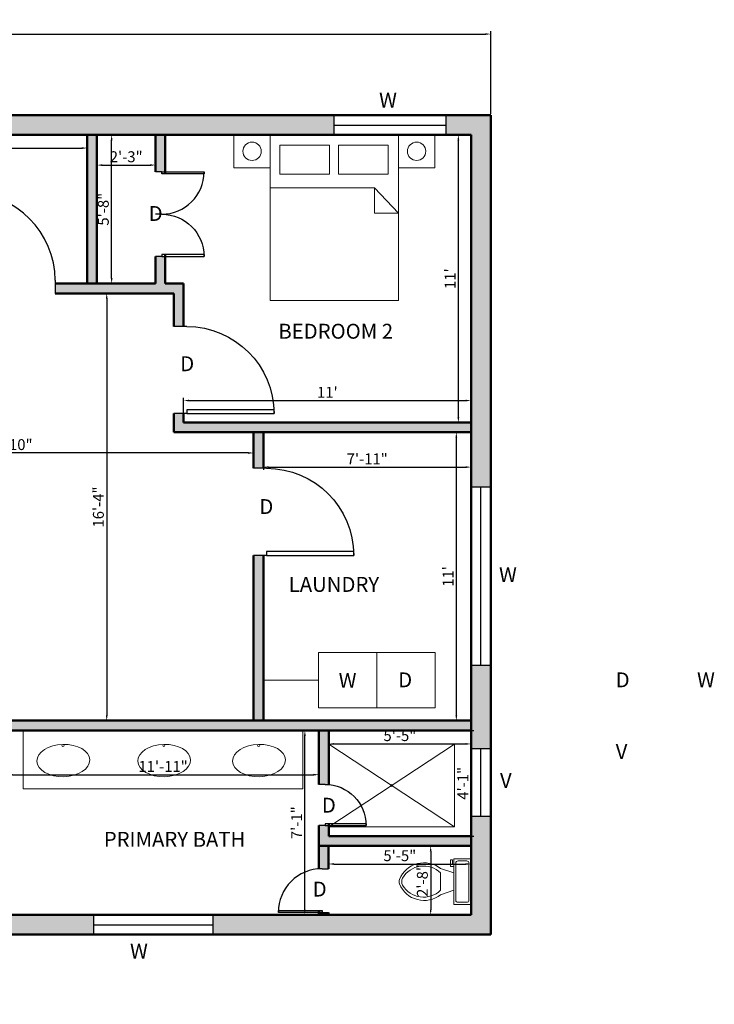
# Model space of a CAD drawing. Units: inches. Extents: x 1838 to 3464, y 573 to 2547.
# Tile 5 of 6: x 3055 to 3374, y 1336 to 1788. Entities that reach past the tile are written whole.
import ezdxf

# ---------------------------------------------------------------- set-up
doc = ezdxf.new("R2010")
doc.units = ezdxf.units.IN
for name, color, linetype, lineweight in [('A-ANNO-DIMS', 2, 'Continuous', 18), ('A-ANNO-TEXT', 7, 'Continuous', 18), ('A-AREA-IDEN', 3, 'Continuous', 18), ('A-DOOR', 4, 'Continuous', 25), ('A-EQPM', 9, 'Continuous', 18), ('A-FLOR-FIXT', 9, 'Continuous', 18), ('A-FURN', 8, 'Continuous', 18), ('A-GLAZ', 3, 'Continuous', 25), ('A-WALL', 1, 'Continuous', 50), ('A-WALL-PATT', 8, 'Continuous', 13)]:
    doc.layers.add(name, color=color, linetype=linetype, lineweight=lineweight)
doc.styles.get("Standard").update_dxf_attribs({"font": 'arial.ttf'})
doc.dimstyles.new('ISO-25', dxfattribs={"dimtxt": 5, "dimasz": 2.5, "dimexe": 1.25, "dimexo": 0.625, "dimtad": 1, "dimdec": 0, "dimlunit": 4, "dimtxsty": 'Standard', "dimcen": 2.5, "dimadec": 0, "dimazin": 0, "dimtfac": 1, "dimtdec": 0, "dimtmove": 0, "dimatfit": 3, "dimfxl": 1, "dimarcsym": 0})

# ---------------------------------------------------------------- blocks, each defined once
blk = doc.blocks.new('*U2')
for p, q in [((0, 0), (0, -6)), ((40, 0), (40, -6))]:
    blk.add_line(p, q)
blk.add_lwpolyline([(0, 0), (0, 40), (1.75, 40), (1.75, 0)], close=True)
blk.add_arc((0, 0), 40, 0, 90)
blk = doc.blocks.new('*U4')
for p, q in [((9.5, -6), (9.5, -2)), ((-10, -8.5), (-8, -8.5)), ((-10, -9.5), (-10, -8.5)), ((-8, -8.5), (-8, -8)), ((-7, -8), (-7, -9.5)), ((-4, -8), (-6, -14)), ((4, -8), (6, -14)), ((-7, -9.5), (-10, -9.5)), ((4, -14), (-4, -14))]:
    blk.add_line(p, q)
blk.add_lwpolyline([(10.5, -8), (10.5, 0), (-10.5, 0), (-10.5, -8)], close=True)
for points in [[(-9.5, -2), (-9.5, -6)], [(8.5, -1), (-8.5, -1)], [(-8.5, -7), (8.5, -7)]]:
    blk.add_lwpolyline(points)
for centre, radius, start, end in [((-8.62, -1.88), 0.884, 81.8699, 188.1301), ((8.62, -1.88), 0.884, 351.8699, 98.1301), ((-8.62, -6.12), 0.884, 171.8699, 278.1301), ((8.62, -6.12), 0.884, 261.8699, 8.1301), ((3.52, -21.58), 12.17, 141.4691, 247.9714), ((4.2, -21.82), 11.33, 136.3677, 238.9468), ((-3.52, -21.58), 12.17, 292.0284, 38.5307), ((-4.2, -21.82), 11.33, 301.053, 43.6321), ((0, -27.88), 4, 245.7318, 294.2682), ((0, -29), 4, 254.8605, 285.1395)]:
    blk.add_arc(centre, radius, start, end)
blk = doc.blocks.new('*D24')
at = {"layer": 'A-ANNO-DIMS', "color": 0, "lineweight": -2, "transparency": 16777216}
for p, q in [((2937.02, 1734.46), (2937.02, 1727.78)), ((3086.23, 1734.46), (3086.23, 1727.78)), ((2939.52, 1729.03), (3083.73, 1729.03))]:
    blk.add_line(p, q, dxfattribs=at)
at = {"layer": 'A-ANNO-DIMS', "color": 0, "lineweight": 100, "transparency": 16777216}
for points in [[(2939.52, 1729.44), (2939.52, 1728.61), (2937.02, 1729.03)], [(3083.73, 1729.44), (3083.73, 1728.61), (3086.23, 1729.03)]]:
    blk.add_solid(points, dxfattribs=at)
at = {"layer": 'Defpoints', "color": 0, "lineweight": 100, "transparency": 16777216}
for p in [(2937.02, 1735.09), (3086.23, 1735.09), (3086.23, 1729.03)]:
    blk.add_point(p, dxfattribs=at)
at = {"layer": 'A-ANNO-DIMS', "color": 0, "transparency": 16777216, "insert": (3011.63, 1732.2), "char_height": 5, "attachment_point": 5}
blk.add_mtext('12\'-5"', dxfattribs=at)
blk = doc.blocks.new('*D26')
at = {"layer": 'A-ANNO-DIMS', "color": 0, "lineweight": -2, "transparency": 16777216}
for p, q in [((3090.73, 1734.46), (3090.73, 1719.96)), ((3117.57, 1734.46), (3117.57, 1719.96)), ((3093.23, 1721.21), (3115.07, 1721.21))]:
    blk.add_line(p, q, dxfattribs=at)
at = {"layer": 'A-ANNO-DIMS', "color": 0, "lineweight": 100, "transparency": 16777216}
for points in [[(3093.23, 1721.63), (3093.23, 1720.79), (3090.73, 1721.21)], [(3115.07, 1721.63), (3115.07, 1720.79), (3117.57, 1721.21)]]:
    blk.add_solid(points, dxfattribs=at)
at = {"layer": 'Defpoints', "color": 0, "lineweight": 100, "transparency": 16777216}
for p in [(3090.73, 1735.09), (3117.57, 1735.09), (3117.57, 1721.21)]:
    blk.add_point(p, dxfattribs=at)
at = {"layer": 'A-ANNO-DIMS', "color": 0, "transparency": 16777216, "insert": (3104.15, 1724.39), "char_height": 5, "attachment_point": 5}
blk.add_mtext('2\'-3"', dxfattribs=at)
blk = doc.blocks.new('*D27')
at = {"layer": 'A-ANNO-DIMS', "color": 0, "lineweight": -2, "transparency": 16777216}
for p, q in [((3130.52, 1603.71), (3130.52, 1614.41)), ((3133.02, 1613.16), (3260.02, 1613.16)), ((3262.52, 1603.71), (3262.52, 1614.41))]:
    blk.add_line(p, q, dxfattribs=at)
at = {"layer": 'A-ANNO-DIMS', "color": 0, "lineweight": 100, "transparency": 16777216}
for points in [[(3133.02, 1613.57), (3133.02, 1612.74), (3130.52, 1613.16)], [(3260.02, 1613.57), (3260.02, 1612.74), (3262.52, 1613.16)]]:
    blk.add_solid(points, dxfattribs=at)
at = {"layer": 'Defpoints', "color": 0, "lineweight": 100, "transparency": 16777216}
for p in [(3262.52, 1613.16), (3130.52, 1603.09), (3262.52, 1603.09)]:
    blk.add_point(p, dxfattribs=at)
at = {"layer": 'A-ANNO-DIMS', "color": 0, "transparency": 16777216, "insert": (3196.52, 1616.29), "char_height": 5, "attachment_point": 5}
blk.add_mtext("11'", dxfattribs=at)
blk = doc.blocks.new('*D28')
at = {"layer": 'A-ANNO-DIMS', "color": 0, "lineweight": -2, "transparency": 16777216}
for p, q in [((3261.9, 1735.09), (3255.42, 1735.09)), ((3256.67, 1605.59), (3256.67, 1732.59)), ((3261.9, 1603.09), (3255.42, 1603.09))]:
    blk.add_line(p, q, dxfattribs=at)
at = {"layer": 'A-ANNO-DIMS', "color": 0, "lineweight": 100, "transparency": 16777216}
for points in [[(3256.25, 1732.59), (3257.09, 1732.59), (3256.67, 1735.09)], [(3256.25, 1605.59), (3257.09, 1605.59), (3256.67, 1603.09)]]:
    blk.add_solid(points, dxfattribs=at)
at = {"layer": 'Defpoints', "color": 0, "lineweight": 100, "transparency": 16777216}
for p in [(3256.67, 1735.09), (3262.52, 1735.09), (3262.52, 1603.09)]:
    blk.add_point(p, dxfattribs=at)
at = {"layer": 'A-ANNO-DIMS', "color": 0, "transparency": 16777216, "insert": (3253.53, 1669.09), "char_height": 5, "attachment_point": 5, "rotation": 90}
blk.add_mtext("11'", dxfattribs=at)
blk = doc.blocks.new('*D29')
at = {"layer": 'A-ANNO-DIMS', "color": 0, "lineweight": -2, "transparency": 16777216}
for p, q in [((3091.36, 1735.09), (3098.71, 1735.09)), ((3097.46, 1669.34), (3097.46, 1732.59)), ((3091.36, 1666.84), (3098.71, 1666.84))]:
    blk.add_line(p, q, dxfattribs=at)
at = {"layer": 'A-ANNO-DIMS', "color": 0, "lineweight": 100, "transparency": 16777216}
for points in [[(3097.05, 1732.59), (3097.88, 1732.59), (3097.46, 1735.09)], [(3097.05, 1669.34), (3097.88, 1669.34), (3097.46, 1666.84)]]:
    blk.add_solid(points, dxfattribs=at)
at = {"layer": 'Defpoints', "color": 0, "lineweight": 100, "transparency": 16777216}
for p in [(3090.73, 1735.09), (3097.46, 1735.09), (3090.73, 1666.84)]:
    blk.add_point(p, dxfattribs=at)
at = {"layer": 'A-ANNO-DIMS', "color": 0, "transparency": 16777216, "insert": (3094.28, 1700.96), "char_height": 5, "attachment_point": 5, "rotation": 90}
blk.add_mtext('5\'-8"', dxfattribs=at)
blk = doc.blocks.new('*D30')
at = {"layer": 'A-ANNO-DIMS', "color": 0, "lineweight": -2, "transparency": 16777216}
for p, q in [((3167.14, 1597.96), (3167.14, 1581.36)), ((3262.52, 1597.96), (3262.52, 1581.36)), ((3169.64, 1582.61), (3260.02, 1582.61))]:
    blk.add_line(p, q, dxfattribs=at)
at = {"layer": 'A-ANNO-DIMS', "color": 0, "lineweight": 100, "transparency": 16777216}
for points in [[(3169.64, 1583.03), (3169.64, 1582.19), (3167.14, 1582.61)], [(3260.02, 1583.03), (3260.02, 1582.19), (3262.52, 1582.61)]]:
    blk.add_solid(points, dxfattribs=at)
at = {"layer": 'Defpoints', "color": 0, "lineweight": 100, "transparency": 16777216}
for p in [(3167.14, 1598.59), (3262.52, 1598.59), (3262.52, 1582.61)]:
    blk.add_point(p, dxfattribs=at)
at = {"layer": 'A-ANNO-DIMS', "color": 0, "transparency": 16777216, "insert": (3214.83, 1585.74), "char_height": 5, "attachment_point": 5}
blk.add_mtext('7\'-11"', dxfattribs=at)
blk = doc.blocks.new('*D31')
at = {"layer": 'A-ANNO-DIMS', "color": 0, "lineweight": -2, "transparency": 16777216}
for p, q in [((3261.9, 1598.59), (3254.49, 1598.59)), ((3255.74, 1596.09), (3255.74, 1468.77)), ((3261.9, 1466.27), (3254.49, 1466.27))]:
    blk.add_line(p, q, dxfattribs=at)
at = {"layer": 'A-ANNO-DIMS', "color": 0, "lineweight": 100, "transparency": 16777216}
for points in [[(3255.33, 1596.09), (3256.16, 1596.09), (3255.74, 1598.59)], [(3255.33, 1468.77), (3256.16, 1468.77), (3255.74, 1466.27)]]:
    blk.add_solid(points, dxfattribs=at)
at = {"layer": 'Defpoints', "color": 0, "lineweight": 100, "transparency": 16777216}
for p in [(3262.52, 1598.59), (3255.74, 1466.27), (3262.52, 1466.27)]:
    blk.add_point(p, dxfattribs=at)
at = {"layer": 'A-ANNO-DIMS', "color": 0, "transparency": 16777216, "insert": (3252.61, 1532.43), "char_height": 5, "attachment_point": 5, "rotation": 90}
blk.add_mtext("11'", dxfattribs=at)
blk = doc.blocks.new('*D32')
at = {"layer": 'A-ANNO-DIMS', "color": 0, "lineweight": -2, "transparency": 16777216}
for p, q in [((3261.9, 1408.74), (3242.71, 1408.74)), ((3243.96, 1406.24), (3243.96, 1379.59)), ((3261.9, 1377.09), (3242.71, 1377.09))]:
    blk.add_line(p, q, dxfattribs=at)
at = {"layer": 'A-ANNO-DIMS', "color": 0, "lineweight": 100, "transparency": 16777216}
for points in [[(3243.55, 1406.24), (3244.38, 1406.24), (3243.96, 1408.74)], [(3243.55, 1379.59), (3244.38, 1379.59), (3243.96, 1377.09)]]:
    blk.add_solid(points, dxfattribs=at)
at = {"layer": 'Defpoints', "color": 0, "lineweight": 100, "transparency": 16777216}
for p in [(3262.52, 1408.74), (3243.96, 1377.09), (3262.52, 1377.09)]:
    blk.add_point(p, dxfattribs=at)
at = {"layer": 'A-ANNO-DIMS', "color": 0, "transparency": 16777216, "insert": (3240.78, 1392.91), "char_height": 5, "attachment_point": 5, "rotation": 90}
blk.add_mtext('2\'-8"', dxfattribs=at)
blk = doc.blocks.new('*D33')
at = {"layer": 'A-ANNO-DIMS', "color": 0, "lineweight": -2, "transparency": 16777216}
for p, q in [((3197.06, 1408.11), (3197.06, 1399.22)), ((3262.52, 1408.11), (3262.52, 1399.22)), ((3199.56, 1400.47), (3260.02, 1400.47))]:
    blk.add_line(p, q, dxfattribs=at)
at = {"layer": 'A-ANNO-DIMS', "color": 0, "lineweight": 100, "transparency": 16777216}
for points in [[(3199.56, 1400.89), (3199.56, 1400.06), (3197.06, 1400.47)], [(3260.02, 1400.89), (3260.02, 1400.06), (3262.52, 1400.47)]]:
    blk.add_solid(points, dxfattribs=at)
at = {"layer": 'Defpoints', "color": 0, "lineweight": 100, "transparency": 16777216}
for p in [(3197.06, 1408.74), (3262.52, 1408.74), (3262.52, 1400.47)]:
    blk.add_point(p, dxfattribs=at)
at = {"layer": 'A-ANNO-DIMS', "color": 0, "transparency": 16777216, "insert": (3229.79, 1403.64), "char_height": 5, "attachment_point": 5}
blk.add_mtext('5\'-5"', dxfattribs=at)
blk = doc.blocks.new('*D34')
at = {"layer": 'A-ANNO-DIMS', "color": 0, "lineweight": -2, "transparency": 16777216}
for p, q in [((3263.15, 1461.77), (3263.77, 1461.77)), ((3262.52, 1415.74), (3262.52, 1459.27)), ((3263.15, 1413.24), (3263.77, 1413.24))]:
    blk.add_line(p, q, dxfattribs=at)
at = {"layer": 'A-ANNO-DIMS', "color": 0, "lineweight": 100, "transparency": 16777216}
for points in [[(3262.11, 1459.27), (3262.94, 1459.27), (3262.52, 1461.77)], [(3262.11, 1415.74), (3262.94, 1415.74), (3262.52, 1413.24)]]:
    blk.add_solid(points, dxfattribs=at)
at = {"layer": 'Defpoints', "color": 0, "lineweight": 100, "transparency": 16777216}
for p in [(3262.52, 1461.77), (3262.52, 1461.77), (3262.52, 1413.24)]:
    blk.add_point(p, dxfattribs=at)
at = {"layer": 'A-ANNO-DIMS', "color": 0, "transparency": 16777216, "insert": (3259.39, 1437.5), "char_height": 5, "attachment_point": 5, "rotation": 90}
blk.add_mtext('4\'-1"', dxfattribs=at)
blk = doc.blocks.new('*D35')
at = {"layer": 'A-ANNO-DIMS', "color": 0, "lineweight": -2, "transparency": 16777216}
for p, q in [((3197.12, 1461.14), (3197.12, 1454.32)), ((3262.52, 1461.14), (3262.52, 1454.32)), ((3199.62, 1455.57), (3260.02, 1455.57))]:
    blk.add_line(p, q, dxfattribs=at)
at = {"layer": 'A-ANNO-DIMS', "color": 0, "lineweight": 100, "transparency": 16777216}
for points in [[(3199.62, 1455.99), (3199.62, 1455.16), (3197.12, 1455.57)], [(3260.02, 1455.99), (3260.02, 1455.16), (3262.52, 1455.57)]]:
    blk.add_solid(points, dxfattribs=at)
at = {"layer": 'Defpoints', "color": 0, "lineweight": 100, "transparency": 16777216}
for p in [(3197.12, 1461.77), (3262.52, 1461.77), (3262.52, 1455.57)]:
    blk.add_point(p, dxfattribs=at)
at = {"layer": 'A-ANNO-DIMS', "color": 0, "transparency": 16777216, "insert": (3229.82, 1458.74), "char_height": 5, "attachment_point": 5}
blk.add_mtext('5\'-5"', dxfattribs=at)
blk = doc.blocks.new('*D36')
at = {"layer": 'A-ANNO-DIMS', "color": 0, "lineweight": -2, "transparency": 16777216}
for p, q in [((3049.57, 1461.14), (3049.57, 1440.21)), ((3192.62, 1461.14), (3192.62, 1440.21)), ((3052.07, 1441.46), (3190.12, 1441.46))]:
    blk.add_line(p, q, dxfattribs=at)
at = {"layer": 'A-ANNO-DIMS', "color": 0, "lineweight": 100, "transparency": 16777216}
for points in [[(3052.07, 1441.87), (3052.07, 1441.04), (3049.57, 1441.46)], [(3190.12, 1441.87), (3190.12, 1441.04), (3192.62, 1441.46)]]:
    blk.add_solid(points, dxfattribs=at)
at = {"layer": 'Defpoints', "color": 0, "lineweight": 100, "transparency": 16777216}
for p in [(3049.57, 1461.77), (3192.62, 1461.77), (3192.62, 1441.46)]:
    blk.add_point(p, dxfattribs=at)
at = {"layer": 'A-ANNO-DIMS', "color": 0, "transparency": 16777216, "insert": (3121.09, 1444.59), "char_height": 5, "attachment_point": 5}
blk.add_mtext('11\'-11"', dxfattribs=at)
blk = doc.blocks.new('*D37')
at = {"layer": 'A-ANNO-DIMS', "color": 0, "lineweight": -2, "transparency": 16777216}
for p, q in [((3191.99, 1461.77), (3184.93, 1461.77)), ((3186.18, 1379.59), (3186.18, 1459.27)), ((3191.99, 1377.09), (3184.93, 1377.09))]:
    blk.add_line(p, q, dxfattribs=at)
at = {"layer": 'A-ANNO-DIMS', "color": 0, "lineweight": 100, "transparency": 16777216}
for points in [[(3185.77, 1459.27), (3186.6, 1459.27), (3186.18, 1461.77)], [(3185.77, 1379.59), (3186.6, 1379.59), (3186.18, 1377.09)]]:
    blk.add_solid(points, dxfattribs=at)
at = {"layer": 'Defpoints', "color": 0, "lineweight": 100, "transparency": 16777216}
for p in [(3186.18, 1461.77), (3192.62, 1461.77), (3192.62, 1377.09)]:
    blk.add_point(p, dxfattribs=at)
at = {"layer": 'A-ANNO-DIMS', "color": 0, "transparency": 16777216, "insert": (3183.05, 1419.43), "char_height": 5, "attachment_point": 5, "rotation": 90}
blk.add_mtext('7\'-1"', dxfattribs=at)
blk = doc.blocks.new('*D50')
at = {"layer": 'A-ANNO-DIMS', "color": 0, "lineweight": -2, "transparency": 16777216}
for p, q in [((2937.02, 1597.96), (2937.02, 1587.86)), ((3162.64, 1597.96), (3162.64, 1587.86)), ((3160.14, 1589.11), (2939.52, 1589.11))]:
    blk.add_line(p, q, dxfattribs=at)
at = {"layer": 'A-ANNO-DIMS', "color": 0, "lineweight": 100, "transparency": 16777216}
for points in [[(2939.52, 1589.52), (2939.52, 1588.69), (2937.02, 1589.11)], [(3160.14, 1589.52), (3160.14, 1588.69), (3162.64, 1589.11)]]:
    blk.add_solid(points, dxfattribs=at)
at = {"layer": 'Defpoints', "color": 0, "lineweight": 100, "transparency": 16777216}
for p in [(2937.02, 1598.59), (3162.64, 1598.59), (2937.02, 1589.11)]:
    blk.add_point(p, dxfattribs=at)
at = {"layer": 'A-ANNO-DIMS', "color": 0, "transparency": 16777216, "insert": (3049.83, 1592.29), "char_height": 5, "attachment_point": 5}
blk.add_mtext('18\'-10"', dxfattribs=at)
blk = doc.blocks.new('*D51')
at = {"layer": 'A-ANNO-DIMS', "color": 0, "lineweight": -2, "transparency": 16777216}
for p, q in [((3125.4, 1662.34), (3093.94, 1662.34)), ((3095.19, 1659.84), (3095.19, 1468.77)), ((3125.4, 1466.27), (3093.94, 1466.27))]:
    blk.add_line(p, q, dxfattribs=at)
at = {"layer": 'A-ANNO-DIMS', "color": 0, "lineweight": 100, "transparency": 16777216}
for points in [[(3094.77, 1659.84), (3095.61, 1659.84), (3095.19, 1662.34)], [(3094.77, 1468.77), (3095.61, 1468.77), (3095.19, 1466.27)]]:
    blk.add_solid(points, dxfattribs=at)
at = {"layer": 'Defpoints', "color": 0, "lineweight": 100, "transparency": 16777216}
for p in [(3126.02, 1662.34), (3095.19, 1466.27), (3126.02, 1466.27)]:
    blk.add_point(p, dxfattribs=at)
at = {"layer": 'A-ANNO-DIMS', "color": 0, "transparency": 16777216, "insert": (3092.01, 1564.3), "char_height": 5, "attachment_point": 5, "rotation": 90}
blk.add_mtext('16\'-4"', dxfattribs=at)
blk = doc.blocks.new('*D65')
at = {"layer": 'A-ANNO-DIMS', "color": 0, "lineweight": -2, "transparency": 16777216}
for p, q in [((2791.52, 1744.71), (2791.52, 1782.6)), ((2794.02, 1781.35), (3269.02, 1781.35)), ((3271.52, 1744.71), (3271.52, 1782.6))]:
    blk.add_line(p, q, dxfattribs=at)
at = {"layer": 'A-ANNO-DIMS', "color": 0, "lineweight": 100, "transparency": 16777216}
for points in [[(2794.02, 1781.77), (2794.02, 1780.94), (2791.52, 1781.35)], [(3269.02, 1781.77), (3269.02, 1780.94), (3271.52, 1781.35)]]:
    blk.add_solid(points, dxfattribs=at)
at = {"layer": 'Defpoints', "color": 0, "lineweight": 100, "transparency": 16777216}
for p in [(3271.52, 1781.35), (2791.52, 1744.09), (3271.52, 1744.09)]:
    blk.add_point(p, dxfattribs=at)
at = {"layer": 'A-ANNO-DIMS', "color": 0, "transparency": 16777216, "insert": (3031.52, 1784.53), "char_height": 5, "attachment_point": 5}
blk.add_mtext("40'", dxfattribs=at)
blk = doc.blocks.new('BED-QUEEN')
for p, q in [((2829.57, 1710.8), (2877.39, 1710.8)), ((2877.39, 1710.8), (2877.39, 1699.19)), ((2888.43, 1699.19), (2877.39, 1710.8)), ((2877.39, 1699.19), (2888.43, 1699.19))]:
    blk.add_line(p, q)
for points in [[(2829.57, 1735.09), (2812.9, 1735.09), (2812.9, 1719.98), (2829.57, 1719.98)], [(2829.57, 1735.09), (2888.43, 1735.09), (2888.43, 1659.13), (2829.57, 1659.13)], [(2905.11, 1735.09), (2888.43, 1735.09), (2888.43, 1719.98), (2905.11, 1719.98)]]:
    blk.add_lwpolyline(points, close=True)
for centre in [(2821.24, 1727.53), (2896.77, 1727.53)]:
    blk.add_circle(centre, 4.22)

msp = doc.modelspace()

# ---------------------------------------------------------------- hatches: boundary and pattern name
at = {"layer": 'A-WALL-PATT'}
h = msp.add_hatch(color=256, dxfattribs=at)
h.dxf.hatch_style = 1
h.paths.add_polyline_path([(2800.52, 1735.09), (2834.76, 1735.09), (2834.76, 1744.09), (2791.52, 1744.09), (2791.52, 1591.27), (2800.52, 1591.27)])
h.paths.add_polyline_path([(2982.96, 1744.09), (2885.93, 1744.09), (2885.93, 1735.09), (2888.43, 1735.09), (2932.52, 1735.09), (2982.96, 1735.09)])
h.paths.add_polyline_path([(3199.72, 1744.09), (3031.52, 1744.09), (3031.52, 1735.09), (3199.72, 1735.09)])
h.paths.add_polyline_path([(3271.52, 1744.09), (3250.89, 1744.09), (3250.89, 1735.09), (3262.52, 1735.09), (3262.52, 1573.47), (3271.52, 1573.47)])
h.paths.add_polyline_path([(3262.52, 1603.09), (3130.52, 1603.09), (3130.52, 1607.14), (3126.02, 1607.14), (3126.02, 1598.59), (3262.52, 1598.59)])
h.paths.add_polyline_path([(3130.52, 1666.84), (3122.07, 1666.84), (3122.07, 1679.27), (3120.48, 1679.27), (3117.57, 1679.27), (3117.57, 1666.84), (3071.52, 1666.84), (3071.52, 1662.34), (3126.02, 1662.34), (3126.02, 1647.14), (3130.52, 1647.14)])
h.paths.add_polyline_path([(3122.07, 1735.09), (3117.57, 1735.09), (3117.57, 1718.07), (3120.48, 1718.07), (3122.07, 1718.07)])
h.paths.add_polyline_path([(3090.73, 1735.09), (3086.23, 1735.09), (3086.23, 1666.84), (3090.73, 1666.84)])
h.paths.add_polyline_path([(3031.52, 1666.84), (2937.02, 1666.84), (2937.02, 1662.34), (3031.52, 1662.34)])
h.paths.add_polyline_path([(2937.02, 1735.09), (2932.52, 1735.09), (2932.52, 1646.12), (2937.02, 1646.12)])
h.paths.add_polyline_path([(2937.02, 1606.12), (2932.52, 1606.12), (2932.52, 1603.09), (2852.18, 1603.09), (2852.18, 1598.59), (2937.02, 1598.59)])
h.paths.add_polyline_path([(2852.18, 1603.09), (2845.88, 1603.09), (2845.88, 1601.49), (2845.88, 1598.59), (2852.18, 1598.59)])
h.paths.add_polyline_path([(2807.08, 1601.49), (2807.08, 1603.09), (2800.52, 1603.09), (2800.52, 1598.59), (2807.08, 1598.59)], flags=17)
h.paths.add_polyline_path([(2937.02, 1598.59), (2932.24, 1598.59), (2932.24, 1570.68), (2937.02, 1570.68)])
h.paths.add_polyline_path([(2800.52, 1513.09), (2800.52, 1533.8), (2791.52, 1533.8), (2791.52, 1336.09), (2852.63, 1336.09), (2852.63, 1345.09), (2840.19, 1345.09), (2823.52, 1345.09), (2800.52, 1345.09)])
h.paths.add_polyline_path([(2807.08, 1472.56), (2807.08, 1475.47), (2800.52, 1475.47), (2800.52, 1470.97), (2807.08, 1470.97)], flags=17)
h.paths.add_polyline_path([(2892.01, 1513.09), (2887.51, 1513.09), (2887.51, 1475.47), (2845.88, 1475.47), (2845.88, 1472.56), (2845.88, 1470.97), (2892.01, 1470.97)])
h.paths.add_polyline_path([(2973.02, 1517.59), (2800.52, 1517.59), (2800.52, 1513.09), (2968.52, 1513.09), (2968.52, 1510.98), (2973.02, 1510.98)])
h.paths.add_polyline_path([(2856.68, 1598.59), (2852.18, 1598.59), (2852.18, 1517.59), (2856.68, 1517.59)])
h.paths.add_polyline_path([(2973.02, 1376.09), (2973.02, 1377.09), (2968.52, 1377.09), (2968.52, 1345.09), (2903.8, 1345.09), (2903.8, 1336.09), (2973.02, 1336.09)])
h.paths.add_polyline_path([(3089.35, 1377.09), (2973.02, 1377.09), (2973.02, 1368.09), (3089.35, 1368.09)])
h.paths.add_polyline_path([(2973.02, 1470.98), (2968.52, 1470.98), (2968.52, 1398.48), (2973.02, 1398.48)])
h.paths.add_polyline_path([(3262.52, 1466.27), (2973.02, 1466.27), (2973.02, 1461.77), (3262.52, 1461.77)])
h.paths.add_polyline_path([(3017.96, 1406), (3045.44, 1406), (3045.44, 1404.8), (3017.93, 1404.8), (3017.93, 1406), (3017.96, 1406, -0.397522), (3045.07, 1432.31), (3045.07, 1461.77), (3049.57, 1461.77), (3049.57, 1432.31), (3045.44, 1432.31, 0.401453)])
h.paths.add_polyline_path([(3049.57, 1404.8), (3045.07, 1404.8), (3045.07, 1402.98), (2973.02, 1402.98), (2973.02, 1398.48), (3049.57, 1398.48)])
h.paths.add_polyline_path([(3271.52, 1422.39), (3262.52, 1422.39), (3262.52, 1377.09), (3143.98, 1377.09), (3143.98, 1368.09), (3271.52, 1368.09)])
h.paths.add_polyline_path([(3271.52, 1491.77), (3262.52, 1491.77), (3262.52, 1453.4), (3271.52, 1453.4)])
h.paths.add_polyline_path([(3167.14, 1542.08), (3162.64, 1542.08), (3162.64, 1466.27), (3167.14, 1466.27)])
h.paths.add_polyline_path([(3167.14, 1598.59), (3162.64, 1598.59), (3162.64, 1582.08), (3167.14, 1582.08)])
h = msp.add_hatch(color=256, dxfattribs=at)
h.dxf.hatch_style = 1
h.paths.add_polyline_path([(3197.12, 1461.77), (3192.62, 1461.77), (3192.62, 1436.99), (3195.45, 1436.99, -0.022103), (3197.12, 1436.92)])
h.paths.add_polyline_path([(3262.52, 1413.24), (3197.12, 1413.24), (3197.12, 1418.11), (3195.45, 1418.11), (3192.62, 1418.11), (3192.62, 1408.74), (3262.52, 1408.74)])
h.paths.add_polyline_path([(3197.06, 1408.74), (3192.62, 1408.74), (3192.62, 1398.28, -0.017972), (3194.06, 1398.33), (3197.06, 1398.33)])
h = msp.add_hatch(color=256, dxfattribs=at)
h.dxf.hatch_style = 1
h.paths.add_polyline_path([(3197.06, 1378.28), (3194.06, 1378.28), (3192.62, 1378.28), (3192.62, 1377.09), (3197.06, 1377.09)])

# ---------------------------------------------------------------- linework, layer by layer
at = {"layer": 'A-EQPM'}
for p, q in [((3219.26, 1472.07), (3219.26, 1497.55)), ((3192.52, 1484.81), (3167.14, 1484.81))]:
    msp.add_line(p, q, dxfattribs=at)
msp.add_lwpolyline([(3192.52, 1472.07), (3246, 1472.07), (3246, 1497.55), (3192.52, 1497.55)], close=True, dxfattribs=at)
at = {"layer": 'A-FLOR-FIXT'}
for p, q in [((3197.12, 1455.49), (3254.92, 1455.49)), ((3197.12, 1417.56), (3254.92, 1455.49)), ((3254.92, 1417.56), (3197.12, 1455.49)), ((3254.92, 1455.49), (3254.92, 1417.56)), ((3254.92, 1417.56), (3197.12, 1417.56))]:
    msp.add_line(p, q, dxfattribs=at)
msp.add_lwpolyline([(3056.84, 1461.77), (3185.21, 1461.77), (3185.21, 1434.97), (3056.84, 1434.97)], close=True, dxfattribs=at)
for centre, radius in [((3075.11, 1454.9), 0.474), ((3121.42, 1454.9), 0.474), ((3164.96, 1454.9), 0.474), ((3226.02, 1436.52), 0.409)]:
    msp.add_circle(centre, radius, dxfattribs=at)
for centre in [(3075.27, 1447.95), (3121.58, 1447.95), (3165.13, 1447.95)]:
    msp.add_ellipse(centre, major_axis=(12.1, 0.29), ratio=0.613887, dxfattribs=at)
at = {"layer": 'A-FURN'}
for points in [[(3174.62, 1730.28), (3197.49, 1730.28), (3197.49, 1716.98), (3174.62, 1716.98)], [(3201.61, 1730.28), (3224.48, 1730.28), (3224.48, 1716.98), (3201.61, 1716.98)]]:
    msp.add_lwpolyline(points, close=True, dxfattribs=at)
at = {"layer": 'A-GLAZ'}
for p, q in [((3199.72, 1739.59), (3250.89, 1739.59)), ((3267.02, 1491.77), (3267.02, 1573.47)), ((3267.02, 1422.39), (3267.02, 1453.4)), ((3089.35, 1372.59), (3143.98, 1372.59))]:
    msp.add_line(p, q, dxfattribs=at)
for points in [[(3199.72, 1744.09), (3250.89, 1744.09), (3250.89, 1735.09), (3199.72, 1735.09)], [(3262.52, 1491.77), (3271.52, 1491.77), (3271.52, 1573.47), (3262.52, 1573.47)], [(3262.52, 1422.39), (3271.52, 1422.39), (3271.52, 1453.4), (3262.52, 1453.4)], [(3143.98, 1368.09), (3089.35, 1368.09), (3089.35, 1377.09), (3143.98, 1377.09)]]:
    msp.add_lwpolyline(points, close=True, dxfattribs=at)
at = {"layer": 'A-WALL'}
for p, q in [((2791.52, 1744.09), (3271.52, 1744.09)), ((3271.52, 1744.09), (3271.52, 1368.09)), ((2800.52, 1735.09), (3262.52, 1735.09)), ((3086.23, 1735.09), (3086.23, 1666.84)), ((3090.73, 1735.09), (3090.73, 1666.84)), ((3117.57, 1718.07), (3117.57, 1735.09)), ((3122.07, 1717.22), (3122.07, 1735.09)), ((3262.52, 1735.09), (3130.52, 1735.09)), ((3262.52, 1735.09), (3262.52, 1377.09)), ((3122.07, 1698.6), (3122.07, 1698.73)), ((3117.57, 1666.84), (3117.57, 1679.27)), ((3122.07, 1666.84), (3122.07, 1680.12)), ((3117.57, 1666.84), (3071.52, 1666.84)), ((3130.52, 1666.84), (3122.07, 1666.84)), ((3130.52, 1666.84), (3130.52, 1647.14)), ((3126.02, 1662.34), (3071.52, 1662.34)), ((3126.02, 1662.34), (3126.02, 1647.14)), ((3126.02, 1607.14), (3126.02, 1598.59)), ((3130.52, 1607.14), (3130.52, 1603.09)), ((3130.52, 1603.09), (3262.52, 1603.09)), ((3126.02, 1598.59), (3262.52, 1598.59)), ((3162.64, 1598.59), (3162.64, 1582.08)), ((3167.14, 1598.59), (3167.14, 1582.08)), ((3162.64, 1542.08), (3162.64, 1466.27)), ((3167.14, 1542.08), (3167.14, 1466.27)), ((2973.02, 1466.27), (3262.52, 1466.27)), ((2973.02, 1461.77), (3262.52, 1461.77)), ((3192.62, 1461.77), (3192.62, 1436.99)), ((3197.12, 1461.77), (3197.12, 1436.92)), ((3197.12, 1455.49), (3197.12, 1455.49)), ((3197.12, 1418.93), (3197.12, 1413.24)), ((3192.62, 1418.11), (3192.62, 1408.74)), ((3197.12, 1413.24), (3262.52, 1413.24)), ((3192.62, 1408.74), (3262.52, 1408.74)), ((3192.62, 1408.74), (3192.62, 1398.28)), ((3197.06, 1408.74), (3197.06, 1398.33)), ((3192.62, 1379.16), (3192.62, 1377.09)), ((3197.06, 1378.28), (3197.06, 1377.09)), ((2973.02, 1377.09), (3262.52, 1377.09)), ((2973.02, 1368.09), (3271.52, 1368.09))]:
    msp.add_line(p, q, dxfattribs=at)

# ---------------------------------------------------------------- block references
at = {"layer": 'A-DOOR'}
for p, xscale, yscale, zscale, rotation in [((3120.48, 1718.07), 0.4849649576214688, 0.4849649576214688, 0.4849649576214688, 270), ((3120.48, 1679.27), -0.4849649576214688, 0.4849649576214688, 0.4849649576214688, 270), ((3195.45, 1418.11), -0.4721246961780511, 0.4721246961780511, 0.4721246961780511, 270), ((3194.06, 1378.28), 0.5010716583969415, 0.5010716583969415, 0.5010716583969415, 90)]:
    msp.add_blockref('*U2', p, dxfattribs=dict(at, xscale=xscale, yscale=yscale, zscale=zscale, rotation=rotation))
msp.add_blockref('*U2', (3031.52, 1668.34), dxfattribs=at)
at = {"layer": 'A-DOOR', "xscale": -1, "rotation": 270}
for p in [(3132.02, 1607.14), (3168.64, 1542.08)]:
    msp.add_blockref('*U2', p, dxfattribs=at)
at = {"layer": 'A-FLOR-FIXT', "rotation": 270}
msp.add_blockref('*U4', (3262.52, 1392.39), dxfattribs=at)
at = {"layer": 'A-FURN'}
msp.add_blockref('BED-QUEEN', (340.72, 0), dxfattribs=at)

# ---------------------------------------------------------------- texts
at = {"layer": 'A-ANNO-TEXT', "char_height": 6.84, "attachment_point": 1}
for s, insert in [('W', (3220.27, 1754.47)), ('D', (3114.46, 1702.42)), ('D', (3128.96, 1633.47)), ('D', (3165.3, 1567.92)), ('W', (3275.34, 1536.67)), ('W', (3201.7, 1488.16)), ('D', (3229.06, 1488.39)), ('D', (3328.92, 1488.39)), ('W', (3366.27, 1488.39)), ('V', (3328.92, 1455.54)), ('V', (3275.79, 1442.26)), ('D', (3194, 1430.87)), ('D', (3189.79, 1392.37)), ('W', (3105.89, 1363.93))]:
    msp.add_mtext_dynamic_manual_height_columns(s, width=95.5762, gutter_width=34.2, heights=[0], dxfattribs=dict(at, insert=insert))
at = {"layer": 'A-AREA-IDEN', "attachment_point": 1}
for s, insert, char_height in [('BEDROOM 2', (3174.03, 1648.38), 6.841), ('LAUNDRY', (3178.78, 1532.2), 6.841), ('PRIMARY BATH', (3093.86, 1415.21), 6.8407)]:
    msp.add_mtext_dynamic_manual_height_columns(s, width=95.5762, gutter_width=34.2, heights=[0], dxfattribs=dict(at, insert=insert, char_height=char_height))

# ---------------------------------------------------------------- dimensions: what is measured, and where the dimension line sits
at = {"layer": 'A-ANNO-DIMS'}
for base, p1, p2, picture, middle in [((3271.52, 1781.35), (2791.52, 1744.09), (3271.52, 1744.09), '*D65', (3031.52, 1784.53)), ((3086.23, 1729.03), (2937.02, 1735.09), (3086.23, 1735.09), '*D24', (3011.63, 1732.2)), ((3117.57, 1721.21), (3090.73, 1735.09), (3117.57, 1735.09), '*D26', (3104.15, 1724.39)), ((3262.52, 1613.16), (3130.52, 1603.09), (3262.52, 1603.09), '*D27', (3196.52, 1616.29)), ((2937.02, 1589.11), (3162.64, 1598.59), (2937.02, 1598.59), '*D50', (3049.83, 1592.29)), ((3262.52, 1582.61), (3167.14, 1598.59), (3262.52, 1598.59), '*D30', (3214.83, 1585.74)), ((3192.62, 1441.46), (3049.57, 1461.77), (3192.62, 1461.77), '*D36', (3121.09, 1444.59)), ((3262.52, 1455.57), (3197.12, 1461.77), (3262.52, 1461.77), '*D35', (3229.82, 1458.74)), ((3262.52, 1400.47), (3197.06, 1408.74), (3262.52, 1408.74), '*D33', (3229.79, 1403.64))]:
    dim = msp.add_linear_dim(base=base, p1=p1, p2=p2, dimstyle='ISO-25', override={"dimclrd": 0, "dimclre": 0, "dimclrt": 0}, dxfattribs=at)
    dim.commit()
    dim.dimension.update_dxf_attribs({"geometry": picture, "text_midpoint": middle})
for base, p1, p2, picture, middle in [((3097.46, 1735.09), (3090.73, 1666.84), (3090.73, 1735.09), '*D29', (3094.28, 1700.96)), ((3256.67, 1735.09), (3262.52, 1603.09), (3262.52, 1735.09), '*D28', (3253.53, 1669.09)), ((3095.19, 1466.27), (3126.02, 1662.34), (3126.02, 1466.27), '*D51', (3092.01, 1564.3)), ((3255.74, 1466.27), (3262.52, 1598.59), (3262.52, 1466.27), '*D31', (3252.61, 1532.43)), ((3186.18, 1461.77), (3192.62, 1377.09), (3192.62, 1461.77), '*D37', (3183.05, 1419.43)), ((3262.52, 1461.77), (3262.52, 1413.24), (3262.52, 1461.77), '*D34', (3259.39, 1437.5)), ((3243.96, 1377.09), (3262.52, 1408.74), (3262.52, 1377.09), '*D32', (3240.78, 1392.91))]:
    dim = msp.add_linear_dim(base=base, p1=p1, p2=p2, angle=90, dimstyle='ISO-25', override={"dimclrd": 0, "dimclre": 0, "dimclrt": 0}, dxfattribs=at)
    dim.commit()
    dim.dimension.update_dxf_attribs({"geometry": picture, "text_midpoint": middle})

doc.saveas('drawing.dxf')
